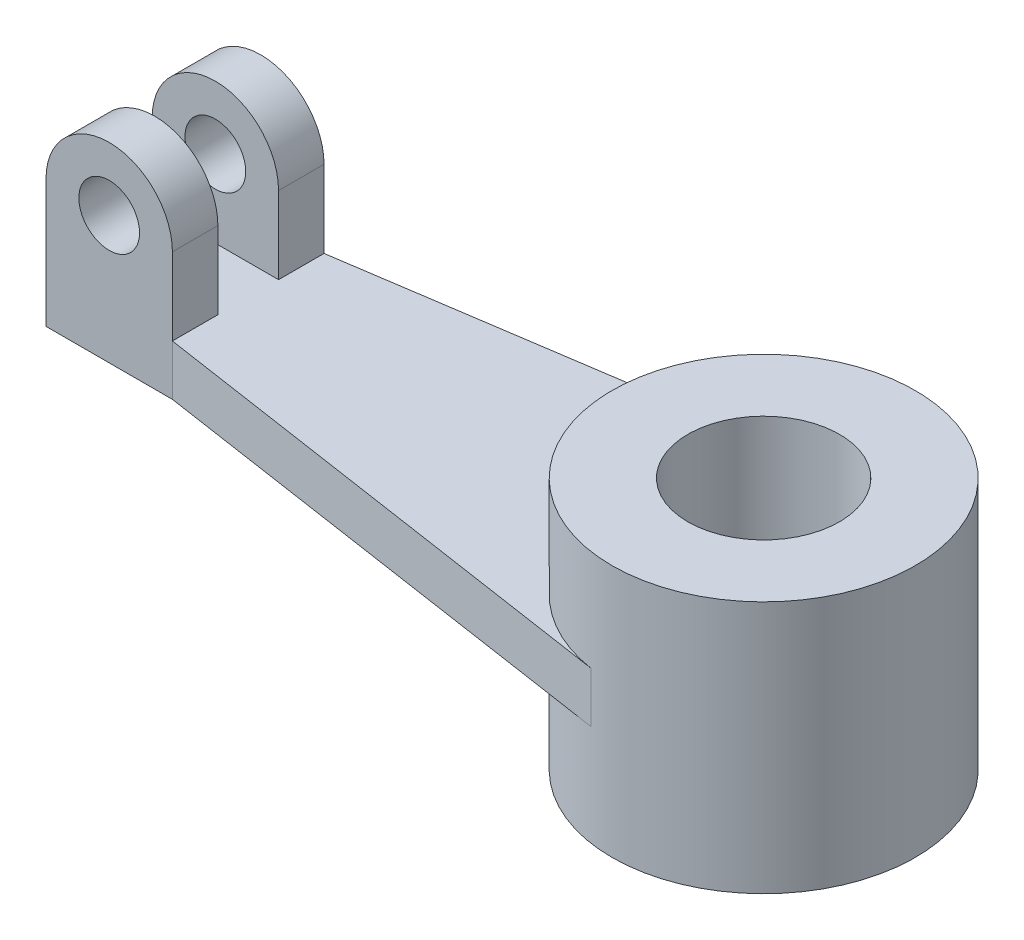
ISO-10303-21;
HEADER;
FILE_DESCRIPTION(('STEP AP214'),'2;1');
FILE_NAME('part.step','',(''),(''),'','','');
FILE_SCHEMA(('AUTOMOTIVE_DESIGN { 1 0 10303 214 1 1 1 1 }'));
ENDSEC;
DATA;
#1=APPLICATION_CONTEXT('core data for automotive mechanical design processes');
#2=APPLICATION_PROTOCOL_DEFINITION('international standard','automotive_design',2000,#1);
#3=PRODUCT_CONTEXT('',#1,'mechanical');
#4=PRODUCT('Part','Part','',(#3));
#5=PRODUCT_RELATED_PRODUCT_CATEGORY('part','',(#4));
#6=PRODUCT_DEFINITION_FORMATION('','',#4);
#7=PRODUCT_DEFINITION_CONTEXT('part definition',#1,'design');
#8=PRODUCT_DEFINITION('design','',#6,#7);
#9=PRODUCT_DEFINITION_SHAPE('','',#8);
#10=(LENGTH_UNIT() NAMED_UNIT(*) SI_UNIT(.MILLI.,.METRE.));
#11=(NAMED_UNIT(*) PLANE_ANGLE_UNIT() SI_UNIT($,.RADIAN.));
#12=(NAMED_UNIT(*) SI_UNIT($,.STERADIAN.) SOLID_ANGLE_UNIT());
#13=UNCERTAINTY_MEASURE_WITH_UNIT(LENGTH_MEASURE(1.E-05),#10,'distance_accuracy_value','');
#14=(GEOMETRIC_REPRESENTATION_CONTEXT(3) GLOBAL_UNCERTAINTY_ASSIGNED_CONTEXT((#13)) GLOBAL_UNIT_ASSIGNED_CONTEXT((#10,
#11,#12)) REPRESENTATION_CONTEXT('',''));
#15=CARTESIAN_POINT('',(0.,0.,0.));
#16=DIRECTION('',(0.,0.,1.));
#17=DIRECTION('',(1.,0.,0.));
#18=AXIS2_PLACEMENT_3D('',#15,#16,#17);
#19=CARTESIAN_POINT('',(0.,5.,0.));
#20=DIRECTION('',(0.,1.,0.));
#21=DIRECTION('',(0.,0.,1.));
#22=AXIS2_PLACEMENT_3D('',#19,#20,#21);
#23=PLANE('',#22);
#24=DIRECTION('',(0.988874898187283,0.,-0.148749573898852));
#25=VECTOR('',#24,1.);
#26=CARTESIAN_POINT('',(-101.962487216966,5.,-15.));
#27=LINE('',#26,#25);
#28=CARTESIAN_POINT('',(-101.962487216966,5.,-15.));
#29=VERTEX_POINT('',#28);
#30=CARTESIAN_POINT('',(-4.46248721696557,5.,-29.6662469456185));
#31=VERTEX_POINT('',#30);
#32=EDGE_CURVE('E209',#29,#31,#27,.T.);
#33=ORIENTED_EDGE('',*,*,#32,.F.);
#34=DIRECTION('',(0.,0.,-1.));
#35=VECTOR('',#34,1.);
#36=CARTESIAN_POINT('',(-101.962487216966,5.,-5.99999999999996));
#37=LINE('',#36,#35);
#38=CARTESIAN_POINT('',(-101.962487216966,5.,-5.99999999999996));
#39=VERTEX_POINT('',#38);
#40=EDGE_CURVE('E57',#39,#29,#37,.T.);
#41=ORIENTED_EDGE('',*,*,#40,.F.);
#42=DIRECTION('',(1.,0.,0.));
#43=VECTOR('',#42,1.);
#44=CARTESIAN_POINT('',(0.,5.,-5.99999999999996));
#45=LINE('',#44,#43);
#46=CARTESIAN_POINT('',(-126.962487216966,5.,-5.99999999999995));
#47=VERTEX_POINT('',#46);
#48=EDGE_CURVE('E58',#47,#39,#45,.T.);
#49=ORIENTED_EDGE('',*,*,#48,.F.);
#50=DIRECTION('',(0.,0.,-1.));
#51=VECTOR('',#50,1.);
#52=CARTESIAN_POINT('',(-126.962487216966,5.,15.));
#53=LINE('',#52,#51);
#54=CARTESIAN_POINT('',(-126.962487216966,5.,6.00000000000003));
#55=VERTEX_POINT('',#54);
#56=EDGE_CURVE('E137',#55,#47,#53,.T.);
#57=ORIENTED_EDGE('',*,*,#56,.F.);
#58=DIRECTION('',(-1.,0.,0.));
#59=VECTOR('',#58,1.);
#60=CARTESIAN_POINT('',(0.,5.,6.00000000000003));
#61=LINE('',#60,#59);
#62=CARTESIAN_POINT('',(-101.962487216966,5.,6.00000000000003));
#63=VERTEX_POINT('',#62);
#64=EDGE_CURVE('E175',#63,#55,#61,.T.);
#65=ORIENTED_EDGE('',*,*,#64,.F.);
#66=DIRECTION('',(0.,0.,1.));
#67=VECTOR('',#66,1.);
#68=CARTESIAN_POINT('',(-101.962487216966,5.,6.00000000000003));
#69=LINE('',#68,#67);
#70=CARTESIAN_POINT('',(-101.962487216966,5.,15.));
#71=VERTEX_POINT('',#70);
#72=EDGE_CURVE('E184',#63,#71,#69,.T.);
#73=ORIENTED_EDGE('',*,*,#72,.T.);
#74=DIRECTION('',(0.988874898187283,0.,0.148749573898851));
#75=VECTOR('',#74,1.);
#76=CARTESIAN_POINT('',(-101.962487216966,5.,15.));
#77=LINE('',#76,#75);
#78=CARTESIAN_POINT('',(-4.46248721696554,5.,29.6662469456185));
#79=VERTEX_POINT('',#78);
#80=EDGE_CURVE('E204',#71,#79,#77,.T.);
#81=ORIENTED_EDGE('',*,*,#80,.T.);
#82=CARTESIAN_POINT('',(0.,5.,0.));
#83=DIRECTION('',(0.,1.,0.));
#84=DIRECTION('',(0.,0.,1.));
#85=AXIS2_PLACEMENT_3D('',#82,#83,#84);
#86=CIRCLE('',#85,30.);
#87=EDGE_CURVE('E210',#31,#79,#86,.T.);
#88=ORIENTED_EDGE('',*,*,#87,.F.);
#89=EDGE_LOOP('',(#33,#41,#49,#57,#65,#73,#81,#88));
#90=FACE_BOUND('',#89,.T.);
#91=ADVANCED_FACE('F41',(#90),#23,.T.);
#92=CARTESIAN_POINT('',(0.,25.,0.));
#93=DIRECTION('',(0.,-1.,0.));
#94=DIRECTION('',(0.,0.,-1.));
#95=AXIS2_PLACEMENT_3D('',#92,#93,#94);
#96=CYLINDRICAL_SURFACE('',#95,30.);
#97=DIRECTION('',(0.,-1.,0.));
#98=VECTOR('',#97,1.);
#99=CARTESIAN_POINT('',(-4.46248721696557,5.,-29.6662469456185));
#100=LINE('',#99,#98);
#101=CARTESIAN_POINT('',(-4.46248721696557,-5.,-29.6662469456185));
#102=VERTEX_POINT('',#101);
#103=EDGE_CURVE('E223',#31,#102,#100,.T.);
#104=ORIENTED_EDGE('',*,*,#103,.F.);
#105=ORIENTED_EDGE('',*,*,#87,.T.);
#106=DIRECTION('',(0.,-1.,0.));
#107=VECTOR('',#106,1.);
#108=CARTESIAN_POINT('',(-4.46248721696555,5.,29.6662469456185));
#109=LINE('',#108,#107);
#110=CARTESIAN_POINT('',(-4.46248721696555,-5.,29.6662469456185));
#111=VERTEX_POINT('',#110);
#112=EDGE_CURVE('E230',#79,#111,#109,.T.);
#113=ORIENTED_EDGE('',*,*,#112,.T.);
#114=CARTESIAN_POINT('',(0.,-5.,0.));
#115=DIRECTION('',(0.,1.,0.));
#116=DIRECTION('',(0.,0.,1.));
#117=AXIS2_PLACEMENT_3D('',#114,#115,#116);
#118=CIRCLE('',#117,30.);
#119=EDGE_CURVE('E216',#102,#111,#118,.T.);
#120=ORIENTED_EDGE('',*,*,#119,.F.);
#121=EDGE_LOOP('',(#104,#105,#113,#120));
#122=FACE_BOUND('',#121,.T.);
#123=CARTESIAN_POINT('',(0.,25.,0.));
#124=DIRECTION('',(0.,1.,0.));
#125=DIRECTION('',(0.,0.,1.));
#126=AXIS2_PLACEMENT_3D('',#123,#124,#125);
#127=CIRCLE('',#126,30.);
#128=CARTESIAN_POINT('',(0.,25.,30.));
#129=VERTEX_POINT('',#128);
#130=EDGE_CURVE('E11',#129,#129,#127,.T.);
#131=ORIENTED_EDGE('',*,*,#130,.F.);
#132=EDGE_LOOP('',(#131));
#133=FACE_BOUND('',#132,.T.);
#134=CARTESIAN_POINT('',(0.,-25.,0.));
#135=DIRECTION('',(0.,1.,0.));
#136=DIRECTION('',(0.,0.,1.));
#137=AXIS2_PLACEMENT_3D('',#134,#135,#136);
#138=CIRCLE('',#137,30.);
#139=CARTESIAN_POINT('',(0.,-25.,30.));
#140=VERTEX_POINT('',#139);
#141=EDGE_CURVE('E44',#140,#140,#138,.T.);
#142=ORIENTED_EDGE('',*,*,#141,.T.);
#143=EDGE_LOOP('',(#142));
#144=FACE_BOUND('',#143,.T.);
#145=ADVANCED_FACE('F43',(#122,#133,#144),#96,.T.);
#146=CARTESIAN_POINT('',(0.,25.,0.));
#147=DIRECTION('',(0.,1.,0.));
#148=DIRECTION('',(0.,0.,1.));
#149=AXIS2_PLACEMENT_3D('',#146,#147,#148);
#150=PLANE('',#149);
#151=CARTESIAN_POINT('',(0.,25.,0.));
#152=DIRECTION('',(0.,1.,0.));
#153=DIRECTION('',(0.,0.,1.));
#154=AXIS2_PLACEMENT_3D('',#151,#152,#153);
#155=CIRCLE('',#154,15.);
#156=CARTESIAN_POINT('',(0.,25.,15.));
#157=VERTEX_POINT('',#156);
#158=EDGE_CURVE('E228',#157,#157,#155,.T.);
#159=ORIENTED_EDGE('',*,*,#158,.F.);
#160=EDGE_LOOP('',(#159));
#161=FACE_BOUND('',#160,.T.);
#162=ORIENTED_EDGE('',*,*,#130,.T.);
#163=EDGE_LOOP('',(#162));
#164=FACE_BOUND('',#163,.T.);
#165=ADVANCED_FACE('F239',(#161,#164),#150,.T.);
#166=CARTESIAN_POINT('',(0.,-25.,0.));
#167=DIRECTION('',(0.,1.,0.));
#168=DIRECTION('',(0.,0.,1.));
#169=AXIS2_PLACEMENT_3D('',#166,#167,#168);
#170=PLANE('',#169);
#171=CARTESIAN_POINT('',(0.,-25.,0.));
#172=DIRECTION('',(0.,1.,0.));
#173=DIRECTION('',(0.,0.,1.));
#174=AXIS2_PLACEMENT_3D('',#171,#172,#173);
#175=CIRCLE('',#174,15.);
#176=CARTESIAN_POINT('',(0.,-25.,15.));
#177=VERTEX_POINT('',#176);
#178=EDGE_CURVE('E233',#177,#177,#175,.T.);
#179=ORIENTED_EDGE('',*,*,#178,.T.);
#180=EDGE_LOOP('',(#179));
#181=FACE_BOUND('',#180,.T.);
#182=ORIENTED_EDGE('',*,*,#141,.F.);
#183=EDGE_LOOP('',(#182));
#184=FACE_BOUND('',#183,.T.);
#185=ADVANCED_FACE('F244',(#181,#184),#170,.F.);
#186=CARTESIAN_POINT('',(0.,-25.,0.));
#187=DIRECTION('',(0.,1.,0.));
#188=DIRECTION('',(0.,0.,1.));
#189=AXIS2_PLACEMENT_3D('',#186,#187,#188);
#190=CYLINDRICAL_SURFACE('',#189,15.);
#191=ORIENTED_EDGE('',*,*,#178,.F.);
#192=EDGE_LOOP('',(#191));
#193=FACE_BOUND('',#192,.T.);
#194=ORIENTED_EDGE('',*,*,#158,.T.);
#195=EDGE_LOOP('',(#194));
#196=FACE_BOUND('',#195,.T.);
#197=ADVANCED_FACE('F240',(#193,#196),#190,.F.);
#198=CARTESIAN_POINT('',(-101.962487216966,5.,15.));
#199=DIRECTION('',(0.148749573898851,0.,-0.988874898187283));
#200=DIRECTION('',(-0.988874898187284,0.,-0.148749573898851));
#201=AXIS2_PLACEMENT_3D('',#198,#199,#200);
#202=PLANE('',#201);
#203=DIRECTION('',(0.988874898187283,0.,0.148749573898851));
#204=VECTOR('',#203,1.);
#205=CARTESIAN_POINT('',(-101.962487216966,-5.,15.));
#206=LINE('',#205,#204);
#207=CARTESIAN_POINT('',(-101.962487216966,-5.,15.));
#208=VERTEX_POINT('',#207);
#209=EDGE_CURVE('E205',#208,#111,#206,.T.);
#210=ORIENTED_EDGE('',*,*,#209,.T.);
#211=ORIENTED_EDGE('',*,*,#112,.F.);
#212=ORIENTED_EDGE('',*,*,#80,.F.);
#213=DIRECTION('',(0.,-1.,0.));
#214=VECTOR('',#213,1.);
#215=CARTESIAN_POINT('',(-101.962487216966,5.,15.));
#216=LINE('',#215,#214);
#217=EDGE_CURVE('E213',#71,#208,#216,.T.);
#218=ORIENTED_EDGE('',*,*,#217,.T.);
#219=EDGE_LOOP('',(#210,#211,#212,#218));
#220=FACE_BOUND('',#219,.T.);
#221=ADVANCED_FACE('F260',(#220),#202,.F.);
#222=CARTESIAN_POINT('',(-101.962487216966,5.,-15.));
#223=DIRECTION('',(-0.148749573898852,0.,-0.988874898187283));
#224=DIRECTION('',(-0.988874898187283,0.,0.148749573898852));
#225=AXIS2_PLACEMENT_3D('',#222,#223,#224);
#226=PLANE('',#225);
#227=DIRECTION('',(0.988874898187283,0.,-0.148749573898852));
#228=VECTOR('',#227,1.);
#229=CARTESIAN_POINT('',(-101.962487216966,-5.,-15.));
#230=LINE('',#229,#228);
#231=CARTESIAN_POINT('',(-101.962487216966,-5.,-15.));
#232=VERTEX_POINT('',#231);
#233=EDGE_CURVE('E208',#232,#102,#230,.T.);
#234=ORIENTED_EDGE('',*,*,#233,.F.);
#235=DIRECTION('',(0.,-1.,0.));
#236=VECTOR('',#235,1.);
#237=CARTESIAN_POINT('',(-101.962487216966,5.,-15.));
#238=LINE('',#237,#236);
#239=EDGE_CURVE('E225',#29,#232,#238,.T.);
#240=ORIENTED_EDGE('',*,*,#239,.F.);
#241=ORIENTED_EDGE('',*,*,#32,.T.);
#242=ORIENTED_EDGE('',*,*,#103,.T.);
#243=EDGE_LOOP('',(#234,#240,#241,#242));
#244=FACE_BOUND('',#243,.T.);
#245=ADVANCED_FACE('F273',(#244),#226,.T.);
#246=CARTESIAN_POINT('',(0.,-5.,0.));
#247=DIRECTION('',(0.,1.,0.));
#248=DIRECTION('',(0.,0.,1.));
#249=AXIS2_PLACEMENT_3D('',#246,#247,#248);
#250=PLANE('',#249);
#251=ORIENTED_EDGE('',*,*,#209,.F.);
#252=DIRECTION('',(-1.,0.,0.));
#253=VECTOR('',#252,1.);
#254=CARTESIAN_POINT('',(-101.962487216966,-5.,15.));
#255=LINE('',#254,#253);
#256=CARTESIAN_POINT('',(-126.962487216966,-5.,15.));
#257=VERTEX_POINT('',#256);
#258=EDGE_CURVE('E198',#208,#257,#255,.T.);
#259=ORIENTED_EDGE('',*,*,#258,.T.);
#260=DIRECTION('',(0.,0.,-1.));
#261=VECTOR('',#260,1.);
#262=CARTESIAN_POINT('',(-126.962487216966,-5.,15.));
#263=LINE('',#262,#261);
#264=CARTESIAN_POINT('',(-126.962487216966,-5.,-15.));
#265=VERTEX_POINT('',#264);
#266=EDGE_CURVE('E195',#257,#265,#263,.T.);
#267=ORIENTED_EDGE('',*,*,#266,.T.);
#268=DIRECTION('',(-1.,0.,0.));
#269=VECTOR('',#268,1.);
#270=CARTESIAN_POINT('',(-101.962487216966,-5.,-15.));
#271=LINE('',#270,#269);
#272=EDGE_CURVE('E193',#232,#265,#271,.T.);
#273=ORIENTED_EDGE('',*,*,#272,.F.);
#274=ORIENTED_EDGE('',*,*,#233,.T.);
#275=ORIENTED_EDGE('',*,*,#119,.T.);
#276=EDGE_LOOP('',(#251,#259,#267,#273,#274,#275));
#277=FACE_BOUND('',#276,.T.);
#278=ADVANCED_FACE('F269',(#277),#250,.F.);
#279=CARTESIAN_POINT('',(-101.962487216966,-5.,15.));
#280=DIRECTION('',(0.,0.,-1.));
#281=DIRECTION('',(-1.,0.,0.));
#282=AXIS2_PLACEMENT_3D('',#279,#280,#281);
#283=PLANE('',#282);
#284=ORIENTED_EDGE('',*,*,#217,.F.);
#285=DIRECTION('',(0.,1.,0.));
#286=VECTOR('',#285,1.);
#287=CARTESIAN_POINT('',(-101.962487216966,0.,15.));
#288=LINE('',#287,#286);
#289=CARTESIAN_POINT('',(-101.962487216966,20.2720523953941,15.));
#290=VERTEX_POINT('',#289);
#291=EDGE_CURVE('E180',#71,#290,#288,.T.);
#292=ORIENTED_EDGE('',*,*,#291,.T.);
#293=CARTESIAN_POINT('',(-114.462487216966,20.2720523953941,15.));
#294=DIRECTION('',(0.,0.,1.));
#295=DIRECTION('',(1.,0.,0.));
#296=AXIS2_PLACEMENT_3D('',#293,#294,#295);
#297=CIRCLE('',#296,12.5);
#298=CARTESIAN_POINT('',(-126.962487216966,20.2720523953941,15.));
#299=VERTEX_POINT('',#298);
#300=EDGE_CURVE('E164',#290,#299,#297,.T.);
#301=ORIENTED_EDGE('',*,*,#300,.T.);
#302=DIRECTION('',(0.,1.,0.));
#303=VECTOR('',#302,1.);
#304=CARTESIAN_POINT('',(-126.962487216966,-5.,15.));
#305=LINE('',#304,#303);
#306=EDGE_CURVE('E199',#257,#299,#305,.T.);
#307=ORIENTED_EDGE('',*,*,#306,.F.);
#308=ORIENTED_EDGE('',*,*,#258,.F.);
#309=EDGE_LOOP('',(#284,#292,#301,#307,#308));
#310=FACE_BOUND('',#309,.T.);
#311=CARTESIAN_POINT('',(-114.462487216966,20.2720523953941,15.));
#312=DIRECTION('',(0.,0.,1.));
#313=DIRECTION('',(1.,0.,0.));
#314=AXIS2_PLACEMENT_3D('',#311,#312,#313);
#315=CIRCLE('',#314,6.);
#316=CARTESIAN_POINT('',(-108.462487216966,20.2720523953941,15.));
#317=VERTEX_POINT('',#316);
#318=EDGE_CURVE('E157',#317,#317,#315,.T.);
#319=ORIENTED_EDGE('',*,*,#318,.F.);
#320=EDGE_LOOP('',(#319));
#321=FACE_BOUND('',#320,.T.);
#322=ADVANCED_FACE('F272',(#310,#321),#283,.F.);
#323=CARTESIAN_POINT('',(-126.962487216966,-5.,15.));
#324=DIRECTION('',(1.,0.,0.));
#325=DIRECTION('',(0.,0.,-1.));
#326=AXIS2_PLACEMENT_3D('',#323,#324,#325);
#327=PLANE('',#326);
#328=ORIENTED_EDGE('',*,*,#306,.T.);
#329=DIRECTION('',(0.,0.,1.));
#330=VECTOR('',#329,1.);
#331=CARTESIAN_POINT('',(-126.962487216966,20.2720523953941,6.00000000000003));
#332=LINE('',#331,#330);
#333=CARTESIAN_POINT('',(-126.962487216966,20.2720523953941,6.00000000000003));
#334=VERTEX_POINT('',#333);
#335=EDGE_CURVE('E189',#334,#299,#332,.T.);
#336=ORIENTED_EDGE('',*,*,#335,.F.);
#337=DIRECTION('',(0.,-1.,0.));
#338=VECTOR('',#337,1.);
#339=CARTESIAN_POINT('',(-126.962487216966,0.,6.00000000000003));
#340=LINE('',#339,#338);
#341=EDGE_CURVE('E172',#334,#55,#340,.T.);
#342=ORIENTED_EDGE('',*,*,#341,.T.);
#343=ORIENTED_EDGE('',*,*,#56,.T.);
#344=DIRECTION('',(0.,-1.,0.));
#345=VECTOR('',#344,1.);
#346=CARTESIAN_POINT('',(-126.962487216966,0.,-5.99999999999996));
#347=LINE('',#346,#345);
#348=CARTESIAN_POINT('',(-126.962487216966,20.2720523953941,-5.99999999999996));
#349=VERTEX_POINT('',#348);
#350=EDGE_CURVE('E138',#349,#47,#347,.T.);
#351=ORIENTED_EDGE('',*,*,#350,.F.);
#352=DIRECTION('',(0.,0.,-1.));
#353=VECTOR('',#352,1.);
#354=CARTESIAN_POINT('',(-126.962487216966,20.2720523953941,-5.99999999999996));
#355=LINE('',#354,#353);
#356=CARTESIAN_POINT('',(-126.962487216966,20.2720523953941,-15.));
#357=VERTEX_POINT('',#356);
#358=EDGE_CURVE('E125',#349,#357,#355,.T.);
#359=ORIENTED_EDGE('',*,*,#358,.T.);
#360=DIRECTION('',(0.,1.,0.));
#361=VECTOR('',#360,1.);
#362=CARTESIAN_POINT('',(-126.962487216966,-5.,-15.));
#363=LINE('',#362,#361);
#364=EDGE_CURVE('E196',#265,#357,#363,.T.);
#365=ORIENTED_EDGE('',*,*,#364,.F.);
#366=ORIENTED_EDGE('',*,*,#266,.F.);
#367=EDGE_LOOP('',(#328,#336,#342,#343,#351,#359,#365,#366));
#368=FACE_BOUND('',#367,.T.);
#369=ADVANCED_FACE('F139',(#368),#327,.F.);
#370=CARTESIAN_POINT('',(-101.962487216966,-5.,-15.));
#371=DIRECTION('',(0.,0.,-1.));
#372=DIRECTION('',(-1.,0.,0.));
#373=AXIS2_PLACEMENT_3D('',#370,#371,#372);
#374=PLANE('',#373);
#375=ORIENTED_EDGE('',*,*,#364,.T.);
#376=CARTESIAN_POINT('',(-114.462487216966,20.2720523953941,-15.));
#377=DIRECTION('',(0.,0.,-1.));
#378=DIRECTION('',(-1.,0.,0.));
#379=AXIS2_PLACEMENT_3D('',#376,#377,#378);
#380=CIRCLE('',#379,12.5);
#381=CARTESIAN_POINT('',(-101.962487216966,20.2720523953941,-15.));
#382=VERTEX_POINT('',#381);
#383=EDGE_CURVE('E128',#357,#382,#380,.T.);
#384=ORIENTED_EDGE('',*,*,#383,.T.);
#385=DIRECTION('',(0.,1.,0.));
#386=VECTOR('',#385,1.);
#387=CARTESIAN_POINT('',(-101.962487216966,0.,-15.));
#388=LINE('',#387,#386);
#389=EDGE_CURVE('E154',#29,#382,#388,.T.);
#390=ORIENTED_EDGE('',*,*,#389,.F.);
#391=ORIENTED_EDGE('',*,*,#239,.T.);
#392=ORIENTED_EDGE('',*,*,#272,.T.);
#393=EDGE_LOOP('',(#375,#384,#390,#391,#392));
#394=FACE_BOUND('',#393,.T.);
#395=CARTESIAN_POINT('',(-114.462487216966,20.2720523953941,-15.));
#396=DIRECTION('',(0.,0.,-1.));
#397=DIRECTION('',(-1.,0.,0.));
#398=AXIS2_PLACEMENT_3D('',#395,#396,#397);
#399=CIRCLE('',#398,6.);
#400=CARTESIAN_POINT('',(-120.462487216966,20.2720523953941,-15.));
#401=VERTEX_POINT('',#400);
#402=EDGE_CURVE('E151',#401,#401,#399,.T.);
#403=ORIENTED_EDGE('',*,*,#402,.F.);
#404=EDGE_LOOP('',(#403));
#405=FACE_BOUND('',#404,.T.);
#406=ADVANCED_FACE('F268',(#394,#405),#374,.T.);
#407=CARTESIAN_POINT('',(-101.962487216966,0.,6.00000000000003));
#408=DIRECTION('',(1.,0.,0.));
#409=DIRECTION('',(0.,0.,-1.));
#410=AXIS2_PLACEMENT_3D('',#407,#408,#409);
#411=PLANE('',#410);
#412=ORIENTED_EDGE('',*,*,#291,.F.);
#413=ORIENTED_EDGE('',*,*,#72,.F.);
#414=DIRECTION('',(0.,1.,0.));
#415=VECTOR('',#414,1.);
#416=CARTESIAN_POINT('',(-101.962487216966,0.,6.00000000000003));
#417=LINE('',#416,#415);
#418=CARTESIAN_POINT('',(-101.962487216966,20.2720523953941,6.00000000000003));
#419=VERTEX_POINT('',#418);
#420=EDGE_CURVE('E163',#63,#419,#417,.T.);
#421=ORIENTED_EDGE('',*,*,#420,.T.);
#422=DIRECTION('',(0.,0.,1.));
#423=VECTOR('',#422,1.);
#424=CARTESIAN_POINT('',(-101.962487216966,20.2720523953941,6.00000000000003));
#425=LINE('',#424,#423);
#426=EDGE_CURVE('E178',#419,#290,#425,.T.);
#427=ORIENTED_EDGE('',*,*,#426,.T.);
#428=EDGE_LOOP('',(#412,#413,#421,#427));
#429=FACE_BOUND('',#428,.T.);
#430=ADVANCED_FACE('F325',(#429),#411,.T.);
#431=CARTESIAN_POINT('',(-114.462487216966,20.2720523953941,6.00000000000003));
#432=DIRECTION('',(0.,0.,1.));
#433=DIRECTION('',(1.,0.,0.));
#434=AXIS2_PLACEMENT_3D('',#431,#432,#433);
#435=CYLINDRICAL_SURFACE('',#434,6.);
#436=CARTESIAN_POINT('',(-114.462487216966,20.2720523953941,6.00000000000003));
#437=DIRECTION('',(0.,0.,1.));
#438=DIRECTION('',(1.,0.,0.));
#439=AXIS2_PLACEMENT_3D('',#436,#437,#438);
#440=CIRCLE('',#439,6.);
#441=CARTESIAN_POINT('',(-108.462487216966,20.2720523953941,6.00000000000003));
#442=VERTEX_POINT('',#441);
#443=EDGE_CURVE('E161',#442,#442,#440,.T.);
#444=ORIENTED_EDGE('',*,*,#443,.F.);
#445=EDGE_LOOP('',(#444));
#446=FACE_BOUND('',#445,.T.);
#447=ORIENTED_EDGE('',*,*,#318,.T.);
#448=EDGE_LOOP('',(#447));
#449=FACE_BOUND('',#448,.T.);
#450=ADVANCED_FACE('F319',(#446,#449),#435,.F.);
#451=CARTESIAN_POINT('',(-114.462487216966,20.2720523953941,6.00000000000003));
#452=DIRECTION('',(0.,0.,1.));
#453=DIRECTION('',(1.,0.,0.));
#454=AXIS2_PLACEMENT_3D('',#451,#452,#453);
#455=CYLINDRICAL_SURFACE('',#454,12.5);
#456=ORIENTED_EDGE('',*,*,#300,.F.);
#457=ORIENTED_EDGE('',*,*,#426,.F.);
#458=CARTESIAN_POINT('',(-114.462487216966,20.2720523953941,6.00000000000003));
#459=DIRECTION('',(0.,0.,1.));
#460=DIRECTION('',(1.,0.,0.));
#461=AXIS2_PLACEMENT_3D('',#458,#459,#460);
#462=CIRCLE('',#461,12.5);
#463=EDGE_CURVE('E169',#419,#334,#462,.T.);
#464=ORIENTED_EDGE('',*,*,#463,.T.);
#465=ORIENTED_EDGE('',*,*,#335,.T.);
#466=EDGE_LOOP('',(#456,#457,#464,#465));
#467=FACE_BOUND('',#466,.T.);
#468=ADVANCED_FACE('F313',(#467),#455,.T.);
#469=CARTESIAN_POINT('',(0.,0.,6.00000000000003));
#470=DIRECTION('',(0.,0.,1.));
#471=DIRECTION('',(1.,0.,0.));
#472=AXIS2_PLACEMENT_3D('',#469,#470,#471);
#473=PLANE('',#472);
#474=ORIENTED_EDGE('',*,*,#443,.T.);
#475=EDGE_LOOP('',(#474));
#476=FACE_BOUND('',#475,.T.);
#477=ORIENTED_EDGE('',*,*,#420,.F.);
#478=ORIENTED_EDGE('',*,*,#64,.T.);
#479=ORIENTED_EDGE('',*,*,#341,.F.);
#480=ORIENTED_EDGE('',*,*,#463,.F.);
#481=EDGE_LOOP('',(#477,#478,#479,#480));
#482=FACE_BOUND('',#481,.T.);
#483=ADVANCED_FACE('F302',(#476,#482),#473,.F.);
#484=CARTESIAN_POINT('',(-101.962487216966,0.,-5.99999999999996));
#485=DIRECTION('',(-1.,0.,0.));
#486=DIRECTION('',(0.,0.,1.));
#487=AXIS2_PLACEMENT_3D('',#484,#485,#486);
#488=PLANE('',#487);
#489=ORIENTED_EDGE('',*,*,#389,.T.);
#490=DIRECTION('',(0.,0.,-1.));
#491=VECTOR('',#490,1.);
#492=CARTESIAN_POINT('',(-101.962487216966,20.2720523953941,-5.99999999999996));
#493=LINE('',#492,#491);
#494=CARTESIAN_POINT('',(-101.962487216966,20.2720523953941,-5.99999999999996));
#495=VERTEX_POINT('',#494);
#496=EDGE_CURVE('E135',#495,#382,#493,.T.);
#497=ORIENTED_EDGE('',*,*,#496,.F.);
#498=DIRECTION('',(0.,1.,0.));
#499=VECTOR('',#498,1.);
#500=CARTESIAN_POINT('',(-101.962487216966,0.,-5.99999999999996));
#501=LINE('',#500,#499);
#502=EDGE_CURVE('E145',#39,#495,#501,.T.);
#503=ORIENTED_EDGE('',*,*,#502,.F.);
#504=ORIENTED_EDGE('',*,*,#40,.T.);
#505=EDGE_LOOP('',(#489,#497,#503,#504));
#506=FACE_BOUND('',#505,.T.);
#507=ADVANCED_FACE('F298',(#506),#488,.F.);
#508=CARTESIAN_POINT('',(-114.462487216966,20.2720523953941,-5.99999999999996));
#509=DIRECTION('',(0.,0.,-1.));
#510=DIRECTION('',(-1.,0.,0.));
#511=AXIS2_PLACEMENT_3D('',#508,#509,#510);
#512=CYLINDRICAL_SURFACE('',#511,6.);
#513=CARTESIAN_POINT('',(-114.462487216966,20.2720523953941,-5.99999999999996));
#514=DIRECTION('',(0.,0.,-1.));
#515=DIRECTION('',(-1.,0.,0.));
#516=AXIS2_PLACEMENT_3D('',#513,#514,#515);
#517=CIRCLE('',#516,6.);
#518=CARTESIAN_POINT('',(-120.462487216966,20.2720523953941,-5.99999999999996));
#519=VERTEX_POINT('',#518);
#520=EDGE_CURVE('E136',#519,#519,#517,.T.);
#521=ORIENTED_EDGE('',*,*,#520,.F.);
#522=EDGE_LOOP('',(#521));
#523=FACE_BOUND('',#522,.T.);
#524=ORIENTED_EDGE('',*,*,#402,.T.);
#525=EDGE_LOOP('',(#524));
#526=FACE_BOUND('',#525,.T.);
#527=ADVANCED_FACE('F304',(#523,#526),#512,.F.);
#528=CARTESIAN_POINT('',(-114.462487216966,20.2720523953941,-5.99999999999996));
#529=DIRECTION('',(0.,0.,-1.));
#530=DIRECTION('',(-1.,0.,0.));
#531=AXIS2_PLACEMENT_3D('',#528,#529,#530);
#532=CYLINDRICAL_SURFACE('',#531,12.5);
#533=ORIENTED_EDGE('',*,*,#383,.F.);
#534=ORIENTED_EDGE('',*,*,#358,.F.);
#535=CARTESIAN_POINT('',(-114.462487216966,20.2720523953941,-5.99999999999996));
#536=DIRECTION('',(0.,0.,-1.));
#537=DIRECTION('',(-1.,0.,0.));
#538=AXIS2_PLACEMENT_3D('',#535,#536,#537);
#539=CIRCLE('',#538,12.5);
#540=EDGE_CURVE('E126',#349,#495,#539,.T.);
#541=ORIENTED_EDGE('',*,*,#540,.T.);
#542=ORIENTED_EDGE('',*,*,#496,.T.);
#543=EDGE_LOOP('',(#533,#534,#541,#542));
#544=FACE_BOUND('',#543,.T.);
#545=ADVANCED_FACE('F127',(#544),#532,.T.);
#546=CARTESIAN_POINT('',(0.,0.,-5.99999999999996));
#547=DIRECTION('',(0.,0.,-1.));
#548=DIRECTION('',(-1.,0.,0.));
#549=AXIS2_PLACEMENT_3D('',#546,#547,#548);
#550=PLANE('',#549);
#551=ORIENTED_EDGE('',*,*,#520,.T.);
#552=EDGE_LOOP('',(#551));
#553=FACE_BOUND('',#552,.T.);
#554=ORIENTED_EDGE('',*,*,#350,.T.);
#555=ORIENTED_EDGE('',*,*,#48,.T.);
#556=ORIENTED_EDGE('',*,*,#502,.T.);
#557=ORIENTED_EDGE('',*,*,#540,.F.);
#558=EDGE_LOOP('',(#554,#555,#556,#557));
#559=FACE_BOUND('',#558,.T.);
#560=ADVANCED_FACE('F142',(#553,#559),#550,.F.);
#561=CLOSED_SHELL('',(#91,#145,#165,#185,#197,#221,#245,#278,#322,#369,#406,#430,#450,#468,#483,
#507,#527,#545,#560));
#562=MANIFOLD_SOLID_BREP('B2',#561);
#563=ADVANCED_BREP_SHAPE_REPRESENTATION('',(#18,#562),#14);
#564=SHAPE_DEFINITION_REPRESENTATION(#9,#563);
ENDSEC;
END-ISO-10303-21;
